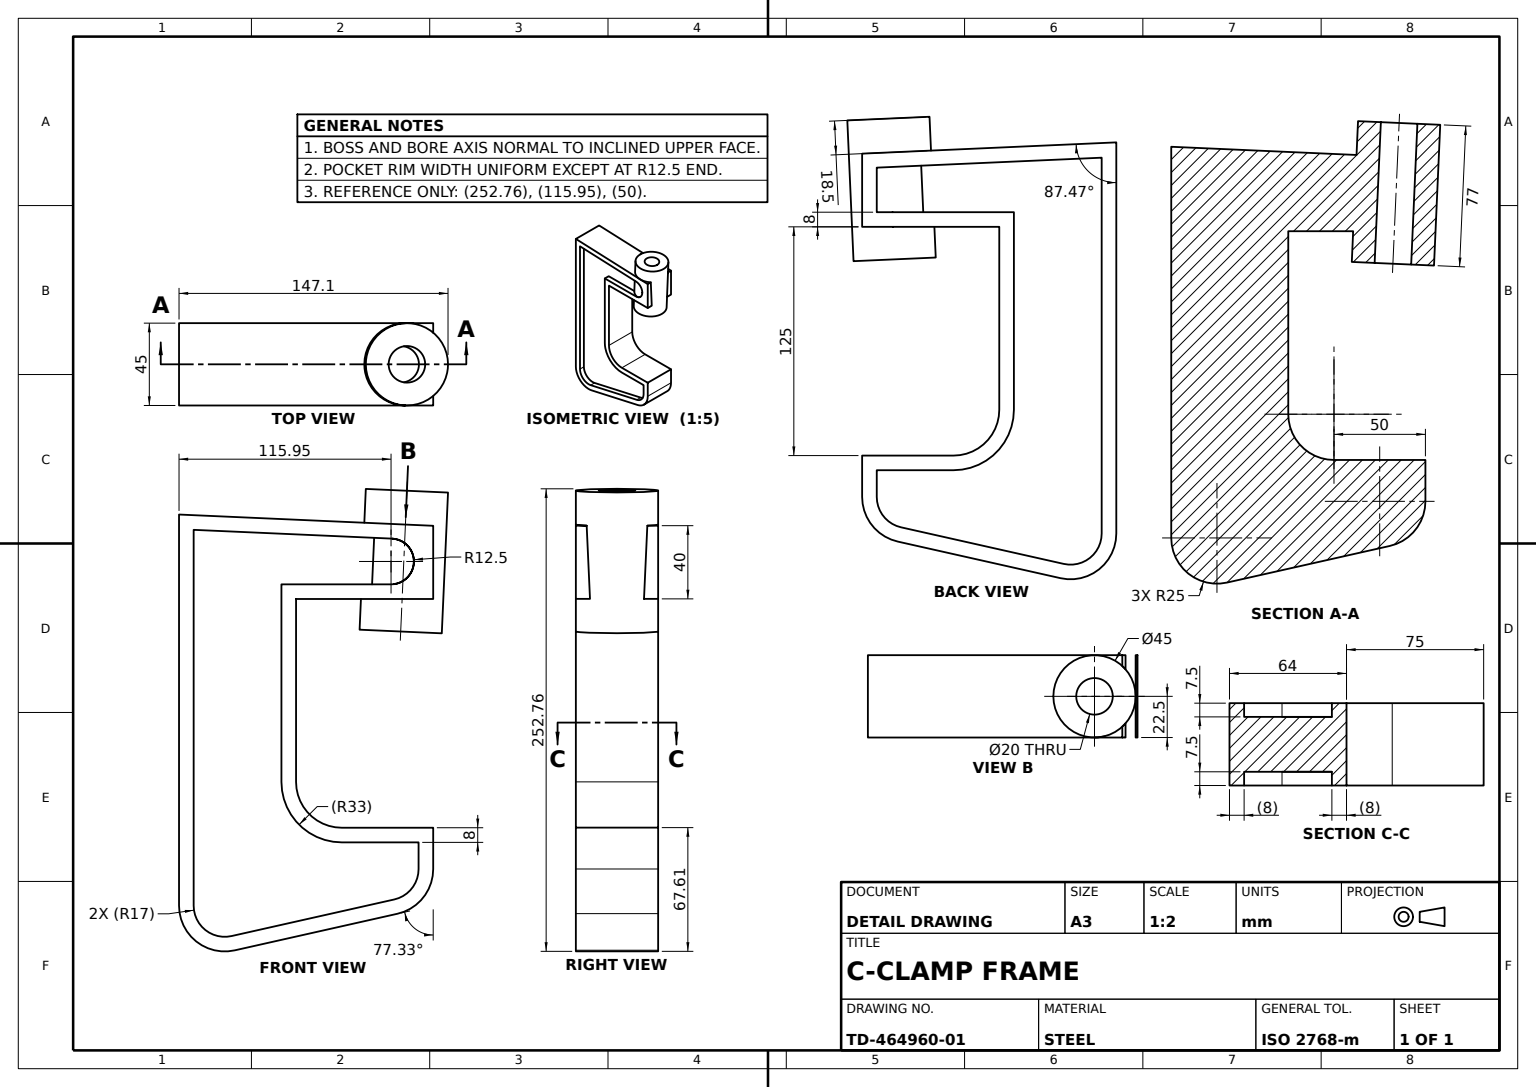
from build123d import *

# Parameters (mm, degrees)
C_FRAME_DEPTH         = 22.5
FRONT_POCKET_DEPTH    = 7.5
BACK_START            = -7.5
BACK_POCKET_DEPTH     = 7.5
SCREW_BOSS_DEPTH      = 18.5
SCREW_BOSS_DEPTH_BACK = 58.5
SCREW_BOSS_SKETCH_R   = 22.5
SCREW_HOLE_SKETCH_R   = 10
SCREW_HOLE_DEPTH      = 98.5


with BuildPart() as part:
    # C Frame Profile Sketch → C Frame (new, symmetric)
    with BuildSketch(Plane.XY):
        with BuildLine():
            Line((108.518716773, 232), (-30.481283227, 238.150273432))
            Line((-30.481283227, 238.150273432), (-30.481283227, 24.391710358))
            ThreePointArc((-30.481283227, 24.391710358), (-21.101269131, 4.872078181), (0, 0))
            Line((0, 0), (89, 20))
            ThreePointArc((89, 20), (103.038348951, 28.771724453), (108.518716773, 44.391710358))
            Line((108.518716773, 44.391710358), (108.518716773, 67))
            Line((108.518716773, 67), (58.518716773, 67))
            ThreePointArc((58.518716773, 67), (40.841047244, 74.32233047), (33.518716773, 92))
            Line((33.518716773, 92), (33.518716773, 192))
            Line((33.518716773, 192), (108.518716773, 192))
            Line((108.518716773, 192), (108.518716773, 232))
        make_face()
    extrude(amount=C_FRAME_DEPTH, both=True)

    # Front Pocket Sketch → Front Pocket (cut)
    with BuildSketch(Plane.XY.offset(22.5)):
        with BuildLine():
            Line((-22.481283227, 229.788473653), (-22.481283227, 24.391710358))
            ThreePointArc((-22.481283227, 24.391710358), (-16.102873642, 11.118360478), (-1.754010632, 7.805347315))
            Line((-1.754010632, 7.805347315), (87.245989368, 27.805347315))
            ThreePointArc((87.245989368, 27.805347315), (96.792066654, 33.770119943), (100.518716773, 44.391710358))
            Line((100.518716773, 44.391710358), (100.518716773, 59))
            Line((100.518716773, 59), (58.518716773, 59))
            ThreePointArc((58.518716773, 59), (35.184192994, 68.665476221), (25.518716773, 92))
            Line((25.518716773, 92), (25.518716773, 200))
            Line((25.518716773, 200), (85.464789993, 200))
            ThreePointArc((85.464789993, 200), (97.961735105, 212.223661697), (86.017331529, 224.987781943))
            Line((86.017331529, 224.987781943), (-22.481283227, 229.788473653))
        make_face()
    extrude(amount=-FRONT_POCKET_DEPTH, mode=Mode.SUBTRACT)

    # Back Pocket Sketch → Back Pocket (cut)
    with BuildSketch(Plane(origin=(0, 0, -22.5), x_dir=(-1, 0, 0), z_dir=(0, 0, -1)).offset(BACK_START)):
        with BuildLine():
            Line((-58.518716773, 59), (-100.518716773, 59))
            Line((-100.518716773, 59), (-100.518716773, 44.391710358))
            ThreePointArc((-100.518716773, 44.391710358), (-96.792066654, 33.770119943), (-87.245989368, 27.805347315))
            Line((-87.245989368, 27.805347315), (1.754010632, 7.805347315))
            ThreePointArc((1.754010632, 7.805347315), (16.102873642, 11.118360478), (22.481283227, 24.391710358))
            Line((22.481283227, 24.391710358), (22.481283227, 229.788473653))
            Line((22.481283227, 229.788473653), (-100.518716773, 224.346145364))
            Line((-100.518716773, 224.346145364), (-100.518716773, 200))
            Line((-100.518716773, 200), (-25.518716773, 200))
            Line((-25.518716773, 200), (-25.518716773, 92))
            ThreePointArc((-25.518716773, 92), (-35.184192994, 68.665476221), (-58.518716773, 59))
        make_face()
    extrude(amount=BACK_POCKET_DEPTH, mode=Mode.SUBTRACT)

    # Screw Boss Sketch → Screw Boss (add, two sides: drawn at the far end of the back side and taken through both)
    with BuildSketch(Plane(origin=(10.457185431, 236.338886554, 0), x_dir=(0.9990225554240701, -0.0442033228837011, 0), z_dir=(0.0442033228837011, 0.9990225554240703, 0)).offset(-SCREW_BOSS_DEPTH_BACK)):
        with Locations(Location((82.951023109, 0, 0), (0, 0, 180))):
            Circle(SCREW_BOSS_SKETCH_R)
    extrude(amount=SCREW_BOSS_DEPTH + SCREW_BOSS_DEPTH_BACK)

    # Screw Hole Sketch → Screw Hole (cut)
    with BuildSketch(Plane(origin=(11.274946905, 254.820803829, 0), x_dir=(0.9990225554240701, -0.04420332288370111, 0), z_dir=(0.04420332288370111, 0.9990225554240703, 0))):
        with Locations(Location((82.951023109, 0, 0), (0, 0, 180))):
            Circle(SCREW_HOLE_SKETCH_R)
    extrude(amount=-SCREW_HOLE_DEPTH, mode=Mode.SUBTRACT)


solid = part.part
